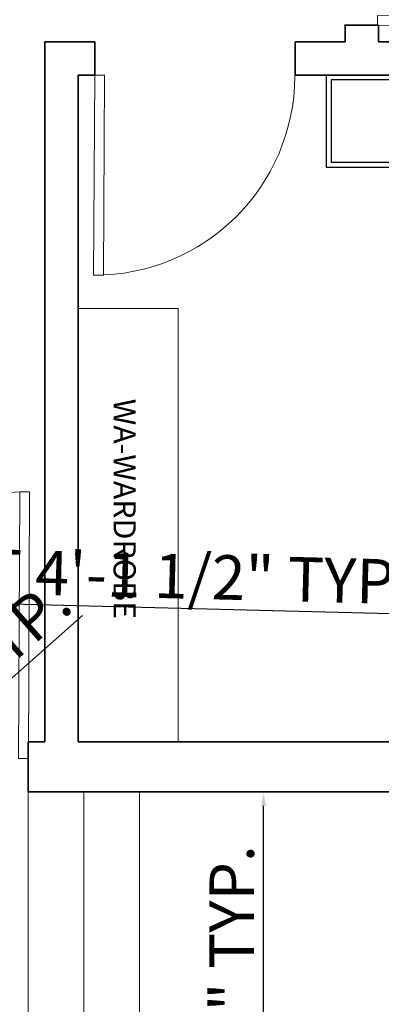
# Model space of a CAD drawing. Units: inches. Extents: x 3394 to 4794, y 965 to 1718.
# Tile 3 of 15: x 3753 to 3818, y 1160 to 1338. Entities that reach past the tile are written whole.
import ezdxf

# ---------------------------------------------------------------- set-up
doc = ezdxf.new("R2010")
doc.units = ezdxf.units.IN
for name, color, linetype, lineweight in [('A-ANNO-DIMS', 2, 'Continuous', 13), ('A-ANNO-TEXT', 7, 'Continuous', 18), ('A-DOOR', 4, 'Continuous', 18), ('A-FLOR-CASE', 8, 'Continuous', 18), ('A-FLOR-STRS', 7, 'Continuous', 18), ('A-WALL', 7, 'Continuous', 35), ('NOITHAT', 21, 'Continuous', 18)]:
    doc.layers.add(name, color=color, linetype=linetype, lineweight=lineweight)
doc.layers.add('FUR', color=42, linetype='Continuous')
doc.styles.get("Standard").update_dxf_attribs({"font": 'arial.ttf'})
doc.dimstyles.new('ISO-25', dxfattribs={"dimtxt": 8, "dimasz": 2.5, "dimexe": 1.25, "dimexo": 0.625, "dimtad": 1, "dimlunit": 3, "dimtxsty": 'Standard', "dimcen": 2.5, "dimadec": 0, "dimazin": 0, "dimtfac": 1, "dimtmove": 0, "dimatfit": 3, "dimfxl": 1, "dimarcsym": 0})

# ---------------------------------------------------------------- blocks, each defined once
blk = doc.blocks.new('*U5')
for p, q in [((0, 0), (0, -6)), ((30, 0), (30, -6))]:
    blk.add_line(p, q)
blk.add_lwpolyline([(0, 0), (0, 30), (1.75, 30), (1.75, 0)], close=True)
blk.add_arc((0, 0), 30, 0, 90)
blk = doc.blocks.new('*U11')
for p, q in [((0, 0), (0, -6)), ((36, 0), (36, -6))]:
    blk.add_line(p, q)
blk.add_lwpolyline([(0, 0), (0, 36), (1.75, 36), (1.75, 0)], close=True)
blk.add_arc((0, 0), 36, 0, 90)
blk = doc.blocks.new('A$C73A16738')
at = {"layer": 'FUR'}
for points in [[(1.428, 0.7893), (2, 0.7893), (2, 0), (1.428, 0)], [(1.458, 0.7593), (1.97, 0.7593), (1.97, 0.03), (1.458, 0.03)]]:
    blk.add_lwpolyline(points, close=True, dxfattribs=at)
blk = doc.blocks.new('DOOR-ENTRY-48IN')
for p, q in [((0.03, 6.2), (0, 0.2)), ((48.03, 6), (48, 0))]:
    blk.add_line(p, q)
blk.add_lwpolyline([(48.03, 6), (48.24, 54), (46.49, 54.01), (46.28, 6.01)], close=True)
blk.add_arc((48.03, 6), 48, 90, 179.759)
blk = doc.blocks.new('STAIR-SITOUT-3STEP')
for p, q in [((129, 68), (129, 20)), ((139, 68), (139, 10)), ((149, 68), (149, 0))]:
    blk.add_line(p, q)
blk = doc.blocks.new('*D73')
at = {"layer": 'A-ANNO-DIMS', "color": 0, "lineweight": -2, "transparency": 16777216}
for p, q in [((3775.37, 1198.68), (3798.34, 1198.68)), ((3797.09, 1133.18), (3797.09, 1196.18)), ((3775.37, 1130.68), (3798.34, 1130.68))]:
    blk.add_line(p, q, dxfattribs=at)
at = {"layer": 'A-ANNO-DIMS', "color": 0, "transparency": 16777216}
for points in [[(3796.68, 1196.18), (3797.51, 1196.18), (3797.09, 1198.68)], [(3796.68, 1133.18), (3797.51, 1133.18), (3797.09, 1130.68)]]:
    blk.add_solid(points, dxfattribs=at)
at = {"layer": 'Defpoints', "color": 0, "transparency": 16777216}
for p in [(3774.74, 1198.68), (3797.09, 1198.68), (3774.74, 1130.68)]:
    blk.add_point(p, dxfattribs=at)
at = {"layer": 'A-ANNO-DIMS', "color": 0, "transparency": 16777216, "insert": (3792.39, 1164.68), "char_height": 8, "attachment_point": 5, "rotation": 90}
blk.add_mtext('5\'-8" TYP.', dxfattribs=at)
blk = doc.blocks.new('*D83')
at = {"layer": 'A-ANNO-DIMS', "color": 0, "lineweight": -2, "transparency": 16777216}
for p, q in [((3707.08, 1179.75), (3764.54, 1230.43)), ((3705.24, 1181.84), (3707.91, 1178.82)), ((3692.13, 1166.56), (3705.21, 1178.1)), ((3688.41, 1167), (3691.08, 1163.97))]:
    blk.add_line(p, q, dxfattribs=at)
at = {"layer": 'A-ANNO-DIMS', "color": 0, "transparency": 16777216}
for points in [[(3704.93, 1178.41), (3705.48, 1177.79), (3707.08, 1179.75)], [(3691.85, 1166.87), (3692.4, 1166.25), (3690.25, 1164.91)]]:
    blk.add_solid(points, dxfattribs=at)
at = {"layer": 'Defpoints', "color": 0, "transparency": 16777216}
for p in [(3704.83, 1182.31), (3707.08, 1179.75), (3687.99, 1167.47)]:
    blk.add_point(p, dxfattribs=at)
at = {"layer": 'A-ANNO-DIMS', "color": 0, "transparency": 16777216, "insert": (3733.6, 1209.49), "char_height": 8, "attachment_point": 5, "rotation": 41.4119}
blk.add_mtext('1\'-10 1/2" TYP.', dxfattribs=at)
blk = doc.blocks.new('*D84')
at = {"layer": 'A-ANNO-DIMS', "color": 0, "lineweight": -2, "transparency": 16777216}
for p, q in [((3828.32, 1230.52), (3710.44, 1233.52)), ((3828.15, 1223.75), (3828.35, 1231.77)), ((3875.11, 1229.33), (3830.82, 1230.46)), ((3877.44, 1222.5), (3877.64, 1230.51))]:
    blk.add_line(p, q, dxfattribs=at)
at = {"layer": 'A-ANNO-DIMS', "color": 0, "transparency": 16777216}
for points in [[(3830.83, 1230.87), (3830.81, 1230.04), (3828.32, 1230.52)], [(3875.12, 1229.75), (3875.1, 1228.91), (3877.61, 1229.27)]]:
    blk.add_solid(points, dxfattribs=at)
at = {"layer": 'Defpoints', "color": 0, "transparency": 16777216}
for p in [(3828.32, 1230.52), (3828.13, 1223.13), (3877.42, 1221.87)]:
    blk.add_point(p, dxfattribs=at)
at = {"layer": 'A-ANNO-DIMS', "color": 0, "transparency": 16777216, "insert": (3768.25, 1236.81), "char_height": 8, "attachment_point": 5, "rotation": 358.5431}
blk.add_mtext('TV UNIT 4\'-1 1/2" TYP.', dxfattribs=at)

msp = doc.modelspace()

# ---------------------------------------------------------------- linework, layer by layer
at = {"layer": 'A-FLOR-CASE'}
for p, q in [((3763.745, 1285.682), (3781.745, 1285.682)), ((3781.745, 1285.682), (3781.745, 1207.682))]:
    msp.add_line(p, q, dxfattribs=at)
at = {"layer": 'A-WALL'}
for p, q in [((3811.745, 1336.682), (3817.745, 1336.682)), ((3811.745, 1336.682), (3811.745, 1333.682)), ((3817.745, 1336.682), (3817.745, 1333.682)), ((3757.745, 1333.682), (3766.745, 1333.682)), ((3757.745, 1333.682), (3757.745, 1207.682)), ((3766.745, 1333.682), (3766.745, 1327.682)), ((3802.745, 1333.682), (3802.745, 1327.682)), ((3802.745, 1333.682), (3811.745, 1333.682)), ((3817.745, 1333.682), (3901.745, 1333.682)), ((3763.745, 1327.682), (3766.745, 1327.682)), ((3763.745, 1327.682), (3763.745, 1207.682)), ((3802.745, 1327.682), (3901.745, 1327.682)), ((3754.745, 1207.682), (3754.745, 1198.682)), ((3754.745, 1207.682), (3757.745, 1207.682)), ((3763.745, 1207.682), (3901.745, 1207.682)), ((3754.745, 1198.682), (3910.745, 1198.682))]:
    msp.add_line(p, q, dxfattribs=at)

# ---------------------------------------------------------------- block references
at = {"layer": 'A-DOOR', "xscale": -1}
for name, p, rotation in [('*U5', (3817.576, 1336.649), 269.6786649249897), ('*U11', (3766.711, 1327.682), 179.6786649249896)]:
    msp.add_blockref(name, p, dxfattribs=dict(at, rotation=rotation))
at = {"layer": 'A-DOOR'}
msp.add_blockref('DOOR-ENTRY-48IN', (3706.745, 1198.682), dxfattribs=at)
at = {"layer": 'A-FLOR-STRS'}
msp.add_blockref('STAIR-SITOUT-3STEP', (3625.745, 1130.682), dxfattribs=at)
at = {"layer": 'NOITHAT', "xscale": -28.92215291203286, "yscale": 28.92215291203286, "zscale": 28.92215291203286, "rotation": 270}
msp.add_blockref('A$C73A16738', (3808.364, 1269.838), dxfattribs=at)

# ---------------------------------------------------------------- texts
at = {"layer": 'A-ANNO-TEXT', "insert": (3774.095, 1269.454), "char_height": 4, "attachment_point": 1, "rotation": 270}
msp.add_mtext_dynamic_manual_height_columns('WA-WARDROBE', width=29.53338, gutter_width=12.5, heights=[0], dxfattribs=at)

# ---------------------------------------------------------------- dimensions: what is measured, and where the dimension line sits
at = {"layer": 'A-ANNO-DIMS'}
for base, p1, p2, angle, text, picture, middle in [((3828.323, 1230.519), (3877.422, 1221.872), (3828.135, 1223.125), 178.54308, 'TV UNIT <> TYP.', '*D84', (3768.252, 1236.809)), ((3707.083, 1179.753), (3687.994, 1167.467), (3704.826, 1182.312), 41.41188, '<> TYP.', '*D83', (3733.601, 1209.491)), ((3797.095, 1198.682), (3774.745, 1130.682), (3774.745, 1198.682), 90, '<> TYP.', '*D73', (3792.385, 1164.682))]:
    dim = msp.add_linear_dim(base=base, p1=p1, p2=p2, angle=angle, text=text, dimstyle='ISO-25', override={"dimdec": 1, "dimlfac": 1, "dimrnd": 0, "dimzin": 1, "dimdsep": 46, "dimlunit": 4, "dimfrac": 2}, dxfattribs=at)
    dim.commit()
    dim.dimension.update_dxf_attribs({"geometry": picture, "text_midpoint": middle})

doc.saveas('drawing.dxf')
